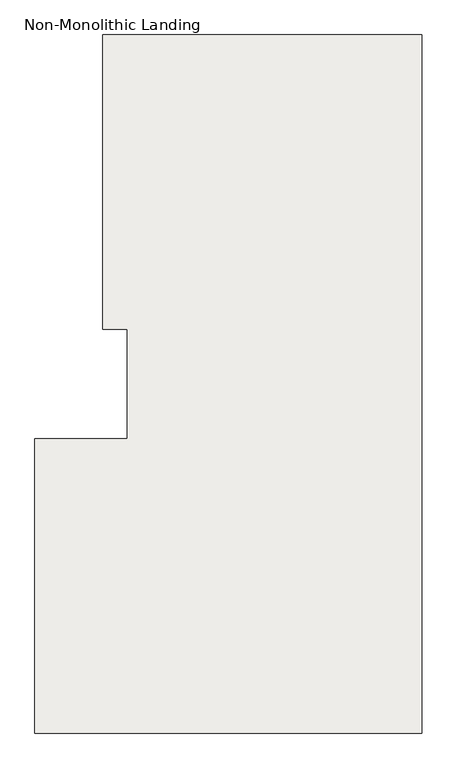
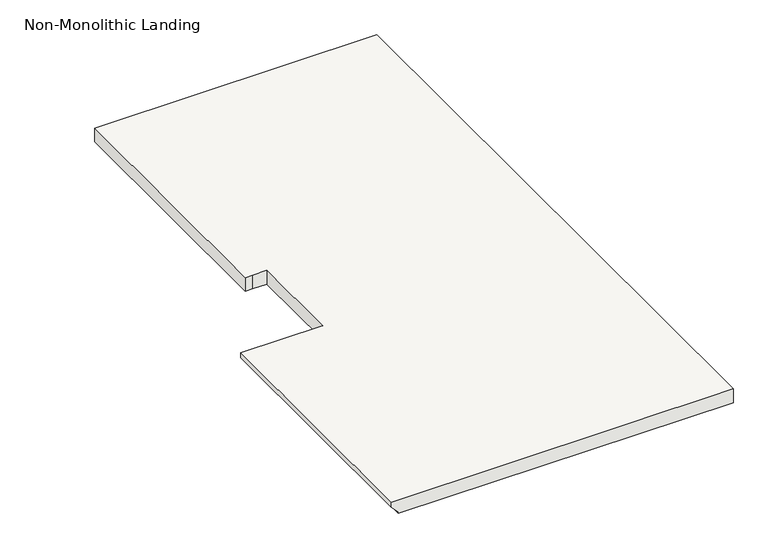
"""IFC4 building model written with IfcOpenShell, lengths in millimetres: slab geometry, Non-Monolithic Landing."""

from ifc_helpers import new_model, si_unit, origin, place, context, project, spatial, faceted_brep, source, transform, mapped, element, save


def non_monolithic_landing_d9a0f4c8(model_context):
    return source(origin(), model_context, "Body", "Brep", [
        faceted_brep([(922.091605, -2823.2158798, 2540.0), (922.091605, -654.9848818, 2540.0), (-43.108395, -654.9848818, 2540.0), (-68.508395, -654.9848818, 2540.0), (-68.508395, -1569.3848818, 2540.0), (-43.108395, -1569.3848818, 2540.0), (7.691605, -1569.3848818, 2540.0), (7.691605, -1908.8158798, 2540.0), (-278.885793, -1908.8158798, 2540.0), (-278.885793, -2823.2158798, 2540.0), (-253.485793, -2823.2158798, 2489.2), (-253.485793, -1908.8158798, 2489.2), (7.691605, -1908.8158798, 2489.2), (7.691605, -1569.3848818, 2489.2), (-43.108395, -1569.3848818, 2489.2), (-68.508395, -1569.3848818, 2489.2), (-68.508395, -654.9848818, 2489.2), (-43.108395, -654.9848818, 2489.2), (922.091605, -654.9848818, 2489.2), (922.091605, -2823.2158798, 2489.2), (-278.885793, -2823.2158798, 2520.95), (-253.485793, -2823.2158798, 2495.55), (-278.885793, -1908.8158798, 2520.95), (-253.485793, -1908.8158798, 2495.55)], [[[0, 1, 2, 3, 4, 5, 6, 7, 8, 9]], [[10, 11, 12, 13, 14, 15, 16, 17, 18, 19]], [[0, 9, 20, 21, 10, 19]], [[1, 0, 19, 18]], [[3, 2, 17, 16]], [[5, 4, 15, 14]], [[6, 5, 14, 13]], [[7, 6, 13, 12]], [[20, 9, 8, 22]], [[21, 20, 22, 23]], [[11, 10, 21, 23]], [[2, 1, 18, 17]], [[4, 3, 16, 15]], [[8, 7, 12, 11, 23, 22]]]),
    ])


if __name__ == "__main__":
    model = new_model("IFC4")
    model_context = context("Model", 3, world=origin())
    ifc_project = project(units=[si_unit("LENGTHUNIT", "METRE", prefix="MILLI")], contexts=[model_context])
    site = spatial("IfcSite", under=ifc_project)
    building = spatial("IfcBuilding", under=site)
    placement = place(None, origin())
    non_monolithic_landing_shape = non_monolithic_landing_d9a0f4c8(model_context)
    element("IfcSlab", 1, ObjectType="Non-Monolithic Landing", at=placement, inside=building, context=model_context, shape_type="MappedRepresentation", body=[
        mapped(non_monolithic_landing_shape, transform((0.0, 0.0, 0.0), x_axis=(1.0, 0.0, 0.0), y_axis=(0.0, 1.0, 0.0), z_axis=(0.0, 0.0, 1.0))),
    ])
    save(model, "model.ifc")
